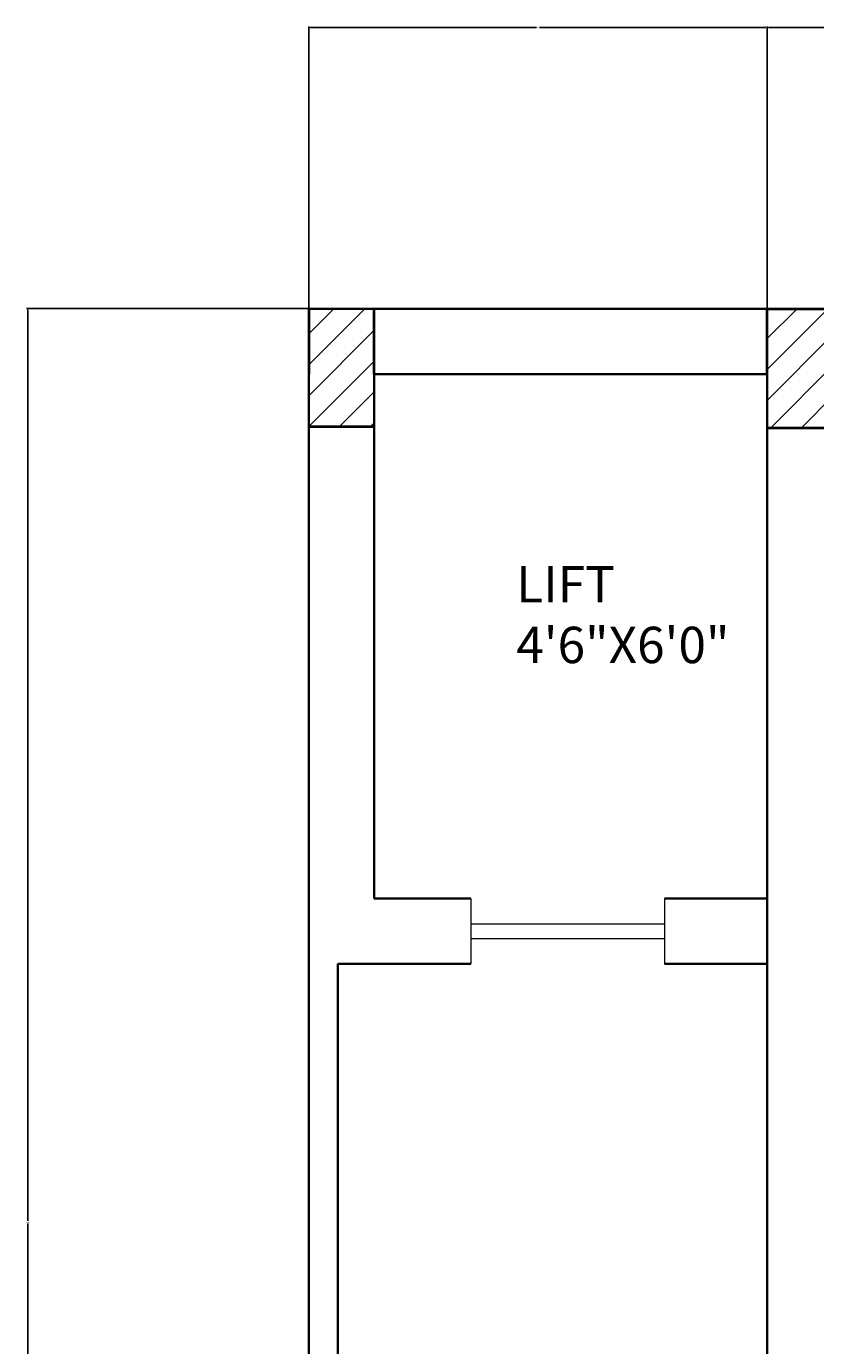
# Model space of a CAD drawing. Units: inches. Extents: x -86 to 2463, y -1058 to 68.
# Tile 12 of 17: x -86 to 22, y -114 to 68. Entities that reach past the tile are written whole.
import ezdxf

# ---------------------------------------------------------------- set-up
doc = ezdxf.new("R2010")
doc.units = ezdxf.units.IN
doc.header["$MEASUREMENT"] = 0
for name, color, linetype, lineweight in [('A-ANNO-DIMS', 2, 'Continuous', 18), ('A-AREA-IDEN', 7, 'Continuous', 18), ('A-COLS', 7, 'Continuous', 40), ('A-COLS-PATT', 252, 'Continuous', 13), ('A-DOOR', 3, 'Continuous', 18), ('A-WALL', 7, 'Continuous', 35)]:
    doc.layers.add(name, color=color, linetype=linetype, lineweight=lineweight)
doc.styles.get("Standard").update_dxf_attribs({"font": 'arial.ttf'})
doc.dimstyles.get("Standard").update_dxf_attribs({"dimtxt": 0.18, "dimasz": 0.18, "dimexe": 0.18, "dimexo": 0.0625, "dimgap": 0.09, "dimtad": 0, "dimtih": 1, "dimtoh": 1, "dimdec": 4, "dimzin": 0, "dimdsep": 46, "dimtxsty": 'Standard', "dimcen": 0.09, "dimadec": 0, "dimazin": 0, "dimtfac": 1, "dimtdec": 4, "dimtofl": 0, "dimtmove": 0, "dimatfit": 3, "dimfxl": 1, "dimtolj": 1, "dimtzin": 0, "dimarcsym": 0})

# ---------------------------------------------------------------- blocks, each defined once
blk = doc.blocks.new('*D32')
at = {"layer": 'A-ANNO-DIMS', "color": 0, "lineweight": -2, "transparency": 16777216}
for p, q in [((15.7, 28.9), (-86.02, 28.9)), ((-85.84, 28.72), (-85.84, -96.42)), ((-85.84, -221.92), (-85.84, -96.79)), ((15.7, -222.1), (-86.02, -222.1))]:
    blk.add_line(p, q, dxfattribs=at)
at = {"layer": 'A-ANNO-DIMS', "color": 0, "transparency": 16777216}
for points in [[(-85.87, 28.72), (-85.81, 28.72), (-85.84, 28.9)], [(-85.87, -221.92), (-85.81, -221.92), (-85.84, -222.1)]]:
    blk.add_solid(points, dxfattribs=at)
at = {"layer": 'Defpoints', "color": 0, "transparency": 16777216}
for p in [(-85.84, 28.9), (15.76, 28.9), (15.76, -222.1)]:
    blk.add_point(p, dxfattribs=at)
at = {"layer": 'A-ANNO-DIMS', "color": 0, "transparency": 16777216, "insert": (-85.84, -96.6), "char_height": 0.18, "attachment_point": 5}
blk.add_mtext('\\A1;251', dxfattribs=at)
blk = doc.blocks.new('*D34')
at = {"layer": 'A-ANNO-DIMS', "color": 0, "lineweight": -2, "transparency": 16777216}
for p, q in [((-47.24, 28.96), (-47.24, 67.68)), ((-47.06, 67.5), (-15.96, 67.5)), ((15.58, 67.5), (-15.52, 67.5)), ((15.76, 28.96), (15.76, 67.68))]:
    blk.add_line(p, q, dxfattribs=at)
at = {"layer": 'A-ANNO-DIMS', "color": 0, "transparency": 16777216}
for points in [[(-47.06, 67.53), (-47.06, 67.47), (-47.24, 67.5)], [(15.58, 67.53), (15.58, 67.47), (15.76, 67.5)]]:
    blk.add_solid(points, dxfattribs=at)
at = {"layer": 'Defpoints', "color": 0, "transparency": 16777216}
for p in [(15.76, 67.5), (-47.24, 28.9), (15.76, 28.9)]:
    blk.add_point(p, dxfattribs=at)
at = {"layer": 'A-ANNO-DIMS', "color": 0, "transparency": 16777216, "insert": (-15.74, 67.5), "char_height": 0.18, "attachment_point": 5}
blk.add_mtext('\\A1;63', dxfattribs=at)
blk = doc.blocks.new('*D35')
at = {"layer": 'A-ANNO-DIMS', "color": 0, "lineweight": -2, "transparency": 16777216}
for p, q in [((15.76, 28.96), (15.76, 67.68)), ((15.94, 67.5), (200.99, 67.5)), ((386.58, 67.5), (201.53, 67.5)), ((386.76, 28.96), (386.76, 67.68))]:
    blk.add_line(p, q, dxfattribs=at)
at = {"layer": 'A-ANNO-DIMS', "color": 0, "transparency": 16777216}
for points in [[(15.94, 67.53), (15.94, 67.47), (15.76, 67.5)], [(386.58, 67.53), (386.58, 67.47), (386.76, 67.5)]]:
    blk.add_solid(points, dxfattribs=at)
at = {"layer": 'Defpoints', "color": 0, "transparency": 16777216}
for p in [(386.76, 67.5), (15.76, 28.9), (386.76, 28.9)]:
    blk.add_point(p, dxfattribs=at)
at = {"layer": 'A-ANNO-DIMS', "color": 0, "transparency": 16777216, "insert": (201.26, 67.5), "char_height": 0.18, "attachment_point": 5}
blk.add_mtext('\\A1;371', dxfattribs=at)

msp = doc.modelspace()

# ---------------------------------------------------------------- hatches: boundary and pattern name
at = {"layer": 'A-COLS-PATT'}
h = msp.add_hatch(dxfattribs=at)
h.set_pattern_fill('ANSI31', color=256, scale=24)
h.set_pattern_definition([(45, (-1015.1314, -586.0864), (-2.1213203, 2.1213203), [])])
h.paths.add_polyline_path([(24.761, -294.104), (24.761, -284.978), (15.761, -284.978), (15.761, -303.104), (24.761, -303.104)])
h.paths.add_polyline_path([(199.1, -294.104), (183.761, -294.104), (183.761, -303.104), (199.1, -303.104)])
h.paths.add_polyline_path([(386.761, -294.104), (377.761, -294.104), (369.914, -294.104), (369.914, -303.104), (377.846, -303.104), (386.761, -303.104)])
h.paths.add_polyline_path([(386.761, -145.104), (386.761, -141.104), (377.761, -141.104), (377.761, -145.104), (377.761, -154.61), (386.761, -154.61)])
h.paths.add_polyline_path([(386.761, -154.61), (377.761, -154.61), (377.761, -162.891), (386.761, -162.891)])
h.paths.add_polyline_path([(24.761, -145.104), (24.761, -141.104), (15.761, -141.104), (15.761, -156.678), (24.761, -156.678)])
h.paths.add_polyline_path([(-38.239, 28.896), (-47.239, 28.896), (-47.239, 19.896), (-47.239, 12.652), (-38.239, 12.652), (-38.239, 19.896)])
h.paths.add_polyline_path([(24.761, 28.896), (15.761, 28.896), (15.761, 19.896), (15.761, 12.545), (24.761, 12.545), (24.761, 19.896)])
h.paths.add_polyline_path([(183.507, 19.896), (161.036, 19.896), (161.036, 17.001), (183.507, 17.001)])
h.paths.add_polyline_path([(183.507, 28.896), (161.036, 28.896), (161.036, 19.896), (183.507, 19.896)])
h.paths.add_polyline_path([(386.761, 28.896), (373.166, 28.896), (373.166, 19.896), (377.761, 19.896), (386.761, 19.896)])

# ---------------------------------------------------------------- linework, layer by layer
at = {"layer": 'A-COLS'}
for p, q in [((-47.239, 28.896), (-47.239, 19.896)), ((-38.239, 19.896), (-38.239, 28.896)), ((15.761, 19.896), (15.761, 28.896)), ((15.761, 28.896), (24.761, 28.896)), ((-38.239, 12.652), (-47.239, 12.652)), ((15.761, 12.545), (24.761, 12.545))]:
    msp.add_line(p, q, dxfattribs=at)
at = {"layer": 'A-DOOR'}
for p, q in [((-24.959, -52.104), (-24.959, -61.104)), ((1.634, -52.104), (1.634, -61.104)), ((-24.959, -55.604), (1.634, -55.604)), ((-24.959, -57.604), (1.634, -57.604))]:
    msp.add_line(p, q, dxfattribs=at)
at = {"layer": 'A-WALL'}
for p, q in [((15.761, 28.896), (-47.239, 28.896)), ((-47.239, -141.104), (-47.239, 19.896)), ((-38.239, -52.104), (-38.239, 19.896)), ((-38.239, 19.896), (15.761, 19.896)), ((15.761, -141.104), (15.761, 19.896)), ((-38.239, -52.104), (-24.959, -52.104)), ((1.634, -52.104), (15.761, -52.104)), ((-43.239, -141.104), (-43.239, -61.104)), ((-38.239, -61.104), (-43.239, -61.104)), ((-38.239, -61.104), (-24.959, -61.104)), ((1.634, -61.104), (15.761, -61.104))]:
    msp.add_line(p, q, dxfattribs=at)

# ---------------------------------------------------------------- texts
at = {"layer": 'A-AREA-IDEN', "insert": (-18.727, -6.46), "char_height": 5, "attachment_point": 1}
msp.add_mtext_dynamic_manual_height_columns('LIFT\\P4\'6"X6\'0"', width=32.82367, gutter_width=25, heights=[0], dxfattribs=at)

# ---------------------------------------------------------------- dimensions: what is measured, and where the dimension line sits
at = {"layer": 'A-ANNO-DIMS'}
for base, p1, p2, picture, middle in [((15.761, 67.496), (-47.239, 28.896), (15.761, 28.896), '*D34', (-15.739, 67.496)), ((386.761, 67.496), (15.761, 28.896), (386.761, 28.896), '*D35', (201.261, 67.496))]:
    dim = msp.add_linear_dim(base=base, p1=p1, p2=p2, dimstyle='Standard', override={"dimdec": 0, "dimlfac": 1, "dimrnd": 0, "dimzin": 0, "dimdsep": 46, "dimlunit": 2}, dxfattribs=at)
    dim.commit()
    dim.dimension.update_dxf_attribs({"geometry": picture, "text_midpoint": middle})
dim = msp.add_linear_dim(base=(-85.839, 28.896), p1=(15.761, -222.104), p2=(15.761, 28.896), angle=90, dimstyle='Standard', override={"dimdec": 0, "dimlfac": 1, "dimrnd": 0, "dimzin": 0, "dimdsep": 46, "dimlunit": 2}, dxfattribs=at)
dim.commit()
dim.dimension.update_dxf_attribs({"geometry": '*D32', "text_midpoint": (-85.839, -96.604)})

doc.saveas('drawing.dxf')
